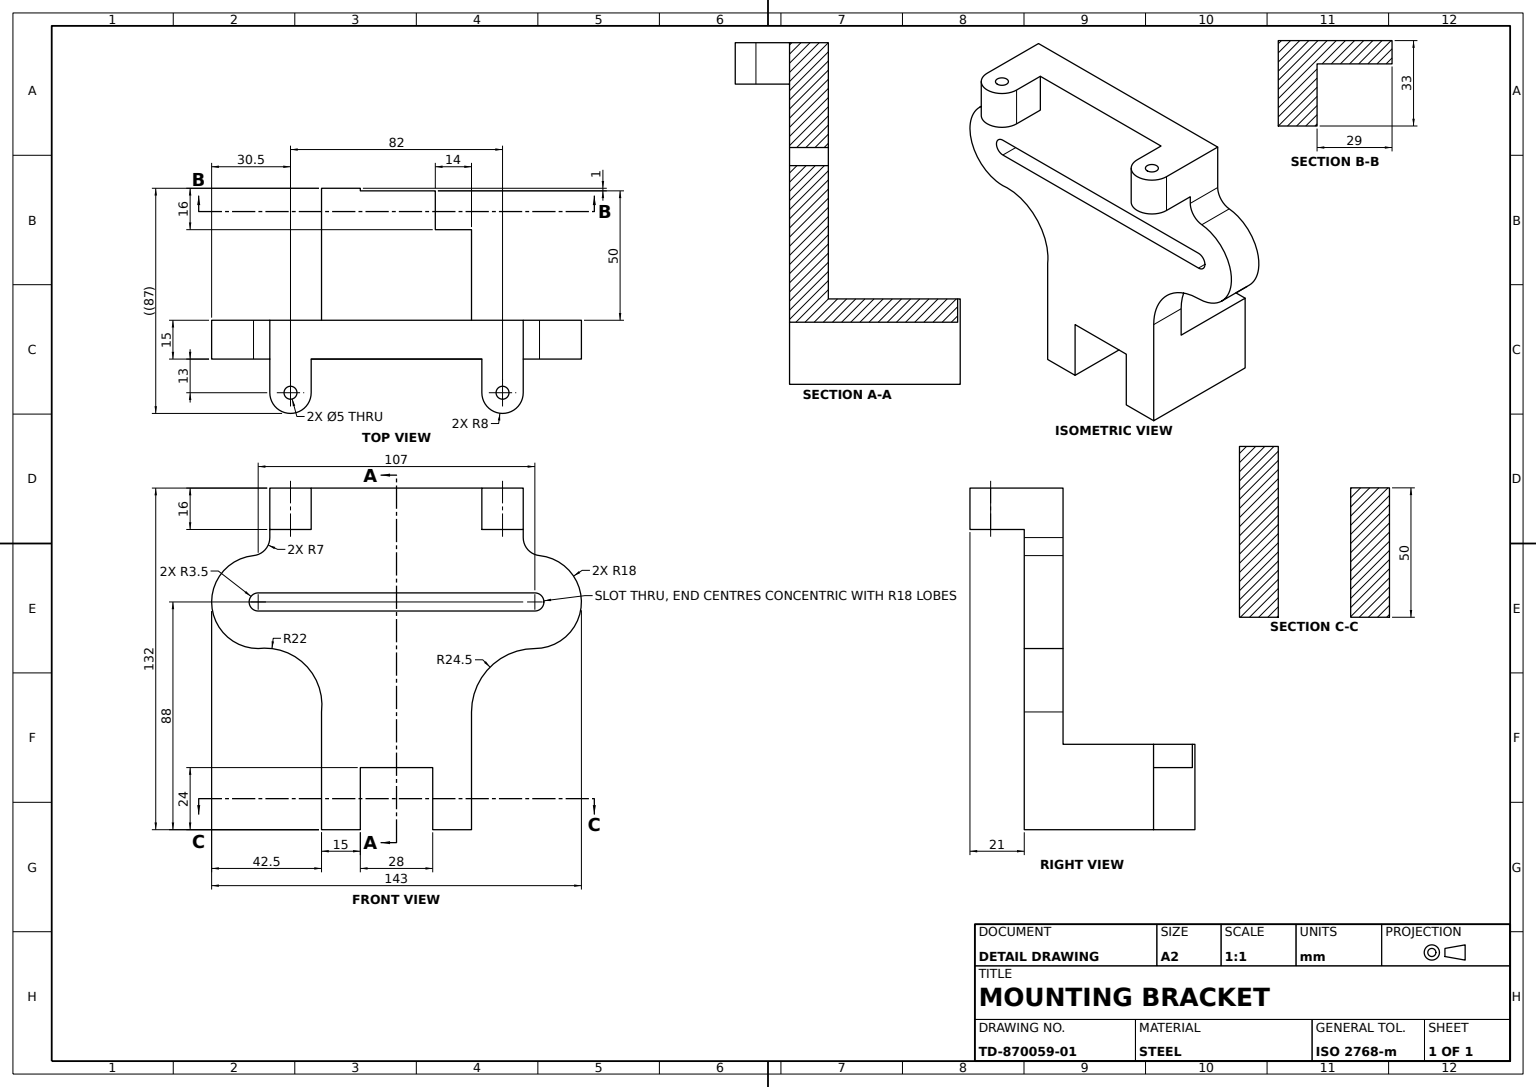
from build123d import *

# Parameters (mm, degrees)
BASE_PLATE_DEPTH         = 15
LONG_SLOT_DEPTH          = 15
LOWER_BLOCK_SKETCH_W     = 66
LOWER_BLOCK_SKETCH_H     = 33
LOWER_BLOCK_33X66_DEPTH  = 15
BLOCK_EXTENSION_SKETCH_W = 29
BLOCK_EXTENSION_SKETCH_H = 9
BLOCK_EXTENSION_DEPTH    = 50
BLOCK_END_SKETCH_W       = 50
BLOCK_END_SKETCH_H       = 33
BLOCK_END_50X50_DEPTH    = 15
LUG_A_DEPTH              = 16
LUG_B_DEPTH              = 16
LUG_HOLES_SKETCH_R       = 2.5
LUG_HOLES_2X5MM_DEPTH    = 16


with BuildPart() as part:
    # Base Plate Profile Sketch → Base Plate (new body)
    with BuildSketch(Plane.XY):
        with BuildLine():
            Line((49, 0), (0, 0))
            Line((0, 0), (0, -19.125314072))
            ThreePointArc((0, -19.125314072), (-1.808661059, -23.821056825), (-6.3, -26.090226132))
            ThreePointArc((-6.3, -26.090226132), (-22.477429316, -44.901129951), (-4.5, -62))
            ThreePointArc((-4.5, -62), (-3.335967318, -61.893154357), (-2.167902709, -61.848286255))
            ThreePointArc((-2.167902709, -61.848286255), (14.519311725, -69.135443097), (20, -86.5))
            Line((20, -86.5), (20, -132))
            Line((20, -132), (34, -132))
            Line((34, -132), (34, -108))
            Line((34, -108), (64, -108))
            Line((64, -108), (64, -132))
            Line((64, -132), (78, -132))
            Line((78, -132), (78, -86.5))
            ThreePointArc((78, -86.5), (85.175883861, -69.175883861), (102.5, -62))
            ThreePointArc((102.5, -62), (120.477429316, -44.901129951), (104.3, -26.090226132))
            ThreePointArc((104.3, -26.090226132), (99.808661059, -23.821056825), (98, -19.125314072))
            Line((98, -19.125314072), (98, 0))
            Line((98, 0), (49, 0))
        make_face()
    extrude(amount=BASE_PLATE_DEPTH)

    # Long Slot Sketch → Long Slot (cut)
    with BuildSketch(Plane.XY.offset(15)):
        with BuildLine():
            Line((-4.5, -40.5), (102.5, -40.5))
            ThreePointArc((102.5, -40.5), (106, -44), (102.5, -47.5))
            Line((102.5, -47.5), (-4.5, -47.5))
            ThreePointArc((-4.5, -47.5), (-8, -44), (-4.5, -40.5))
        make_face()
    extrude(amount=-LONG_SLOT_DEPTH, mode=Mode.SUBTRACT)

    # Lower Block Sketch → Lower Block 33x66 (add)
    with BuildSketch(Plane.ZY.offset(-20)):
        with Locations((-18, -115.5)):
            Rectangle(LOWER_BLOCK_SKETCH_W, LOWER_BLOCK_SKETCH_H)
    extrude(amount=-LOWER_BLOCK_33X66_DEPTH)

    # Block Extension Sketch → Block Extension (add)
    with BuildSketch(Plane(origin=(0, 0, 0), x_dir=(-1, 0, 0), z_dir=(0, 0, -1))):
        with Locations((-49.5, -103.5)):
            Rectangle(BLOCK_EXTENSION_SKETCH_W, BLOCK_EXTENSION_SKETCH_H)
    extrude(amount=BLOCK_EXTENSION_DEPTH)

    # Block End Sketch → Block End 50x50 (add)
    with BuildSketch(Plane(origin=(78, 0, 0), x_dir=(0, 0, -1), z_dir=(1, 0, 0))):
        with Locations((10, -115.5)):
            Rectangle(BLOCK_END_SKETCH_W, BLOCK_END_SKETCH_H)
    extrude(amount=-BLOCK_END_50X50_DEPTH)

    # Lug A Sketch → Lug A (add)
    with BuildSketch(Plane(origin=(0, 0, 0), x_dir=(1, 0, 0), z_dir=(0, 1, 0))):
        with BuildLine():
            Line((8, -15), (0, -15))
            Line((0, -15), (0, -28))
            ThreePointArc((0, -28), (8, -36), (16, -28))
            Line((16, -28), (16, -15))
            Line((16, -15), (8, -15))
        make_face()
    extrude(amount=-LUG_A_DEPTH)

    # Lug B Sketch → Lug B (add)
    with BuildSketch(Plane(origin=(0, 0, 0), x_dir=(1, 0, 0), z_dir=(0, 1, 0))):
        with BuildLine():
            Line((98, -28), (98, -15))
            Line((98, -15), (90, -15))
            Line((90, -15), (82, -15))
            Line((82, -15), (82, -28))
            ThreePointArc((82, -28), (90, -36), (98, -28))
        make_face()
    extrude(amount=-LUG_B_DEPTH)

    # Lug Holes Sketch → Lug Holes 2x5mm (cut)
    with BuildSketch(Plane.XZ.offset(16)):
        with Locations(Location((90, 28, 0), (0, 0, 270))):
            Circle(LUG_HOLES_SKETCH_R)
        with Locations(Location((8, 28, 0), (0, 0, 270))):
            Circle(LUG_HOLES_SKETCH_R)
    extrude(amount=-LUG_HOLES_2X5MM_DEPTH, mode=Mode.SUBTRACT)


solid = part.part
